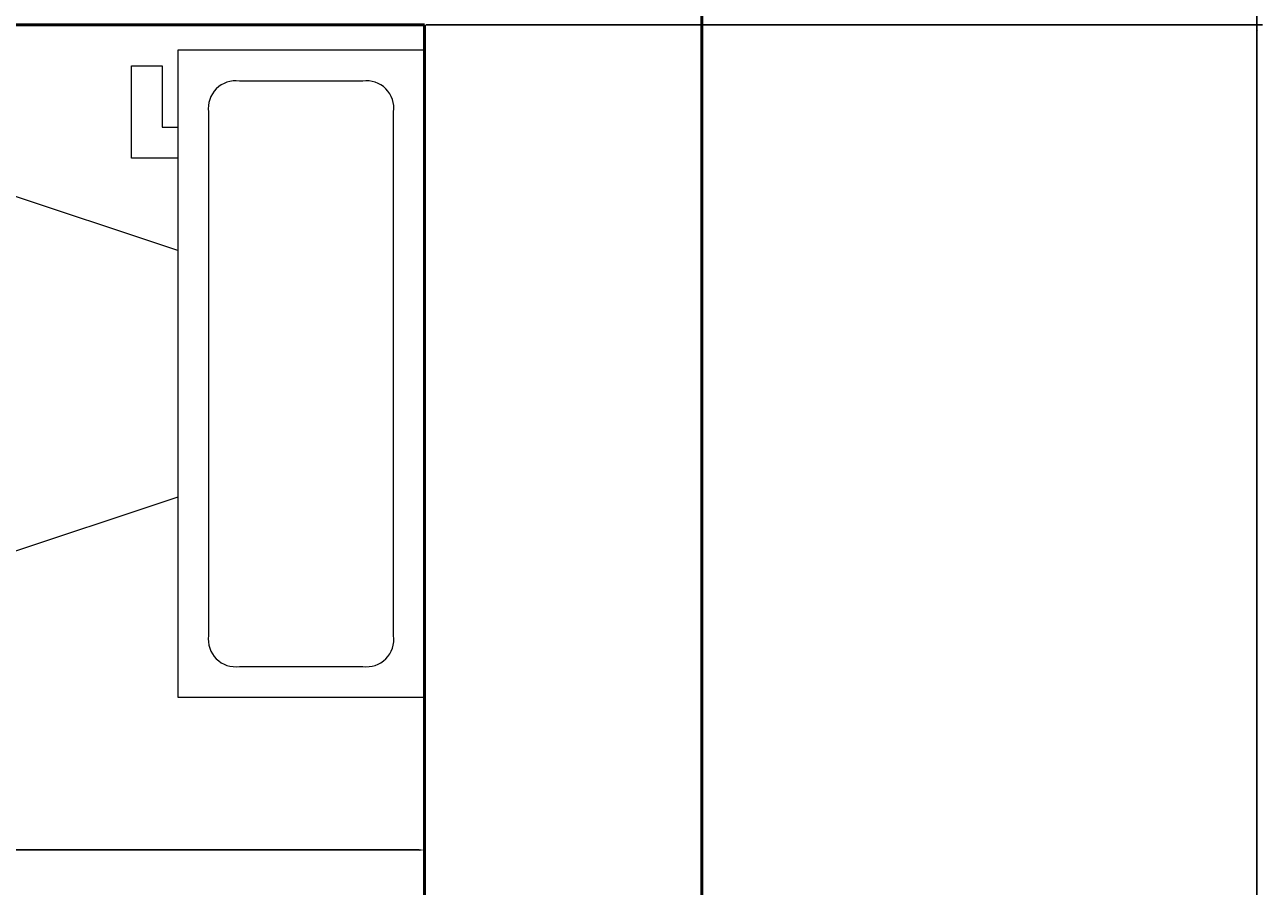
# Model space of a CAD drawing. Units: inches. Extents: x 2621 to 2849, y 2066 to 2463.
# Tile 27 of 28: x 2809 to 2849, y 2407 to 2435. Entities that reach past the tile are written whole.
import ezdxf

# ---------------------------------------------------------------- set-up
doc = ezdxf.new("R2010")
doc.units = ezdxf.units.IN
for name, color, linetype, lineweight in [('A-ANNO-DIMS', 2, 'Continuous', 18), ('A-FLOR-FIXT', 9, 'Continuous', 18), ('A-WALL', 7, 'Continuous', 50)]:
    doc.layers.add(name, color=color, linetype=linetype, lineweight=lineweight)
doc.styles.get("Standard").update_dxf_attribs({"font": 'arial.ttf'})
doc.dimstyles.get("Standard").update_dxf_attribs({"dimtxt": 0.18, "dimasz": 0.18, "dimexe": 0.18, "dimexo": 0.0625, "dimgap": 0.09, "dimtad": 0, "dimtih": 1, "dimtoh": 1, "dimdec": 4, "dimzin": 0, "dimdsep": 46, "dimtxsty": 'Standard', "dimcen": 0.09, "dimadec": 0, "dimazin": 0, "dimtfac": 1, "dimtdec": 4, "dimtofl": 0, "dimtmove": 0, "dimatfit": 3, "dimfxl": 1, "dimtolj": 1, "dimtzin": 0, "dimarcsym": 0})

# ---------------------------------------------------------------- blocks, each defined once
blk = doc.blocks.new('Toilet - top')
for p, q in [((9.5, -6), (9.5, -2)), ((-8, -8.5), (-8, -8)), ((-7, -8), (-7, -9.5)), ((-4, -8), (-6, -14)), ((4, -8), (6, -14)), ((-10, -8.5), (-8, -8.5)), ((-10, -9.5), (-10, -8.5)), ((-7, -9.5), (-10, -9.5)), ((4, -14), (-4, -14))]:
    blk.add_line(p, q)
blk.add_lwpolyline([(10.5, -8), (10.5, 0), (-10.5, 0), (-10.5, -8)], close=True)
for points in [[(8.5, -1), (-8.5, -1)], [(-9.5, -2), (-9.5, -6)], [(-8.5, -7), (8.5, -7)]]:
    blk.add_lwpolyline(points)
for centre, radius, start, end in [((-8.625, -1.875), 0.884, 81.8699, 188.1301), ((8.625, -1.875), 0.884, 351.8699, 98.1301), ((-8.625, -6.125), 0.884, 171.8699, 278.1301), ((8.625, -6.125), 0.884, 261.8699, 8.1301), ((3.52, -21.58), 12.169, 141.4691, 247.9714), ((4.2, -21.817), 11.329, 136.3677, 238.9468), ((-3.519, -21.58), 12.169, 292.0284, 38.5307), ((-4.2, -21.817), 11.329, 301.053, 43.6321), ((0, -27.876), 4, 245.7318, 294.2682), ((0, -29), 4, 254.8605, 285.1395)]:
    blk.add_arc(centre, radius, start, end)
blk = doc.blocks.new('*D27')
at = {"layer": 'A-ANNO-DIMS', "color": 0, "lineweight": -2, "transparency": 16777216}
for p, q in [((2788.824, 2413.484), (2788.824, 2408.409)), ((2821.87, 2413.484), (2821.87, 2408.409)), ((2789.004, 2408.589), (2804.88, 2408.589)), ((2821.69, 2408.589), (2805.814, 2408.589))]:
    blk.add_line(p, q, dxfattribs=at)
at = {"layer": 'A-ANNO-DIMS', "color": 0, "transparency": 16777216}
for points in [[(2789.004, 2408.619), (2789.004, 2408.559), (2788.824, 2408.589)], [(2821.69, 2408.619), (2821.69, 2408.559), (2821.87, 2408.589)]]:
    blk.add_solid(points, dxfattribs=at)
at = {"layer": 'Defpoints', "color": 0, "transparency": 16777216}
for p in [(2788.824, 2413.546), (2821.87, 2413.546), (2821.87, 2408.589)]:
    blk.add_point(p, dxfattribs=at)
at = {"layer": 'A-ANNO-DIMS', "color": 0, "transparency": 16777216, "insert": (2805.347, 2408.589), "char_height": 0.18, "attachment_point": 5}
blk.add_mtext('\\A1;WC 33', dxfattribs=at)
blk = doc.blocks.new('*D36')
at = {"layer": 'A-ANNO-DIMS', "color": 0, "lineweight": -2, "transparency": 16777216}
for p, q in [((2830.933, 2444.375), (2849.054, 2444.375)), ((2848.874, 2444.195), (2848.874, 2264.557)), ((2848.874, 2084.555), (2848.874, 2264.193)), ((2830.933, 2084.375), (2849.054, 2084.375))]:
    blk.add_line(p, q, dxfattribs=at)
at = {"layer": 'A-ANNO-DIMS', "color": 0, "transparency": 16777216}
for points in [[(2848.844, 2444.195), (2848.904, 2444.195), (2848.874, 2444.375)], [(2848.844, 2084.555), (2848.904, 2084.555), (2848.874, 2084.375)]]:
    blk.add_solid(points, dxfattribs=at)
at = {"layer": 'Defpoints', "color": 0, "transparency": 16777216}
for p in [(2830.87, 2444.375), (2848.874, 2444.375), (2830.87, 2084.375)]:
    blk.add_point(p, dxfattribs=at)
at = {"layer": 'A-ANNO-DIMS', "color": 0, "transparency": 16777216, "insert": (2848.874, 2264.375), "char_height": 0.18, "attachment_point": 5}
blk.add_mtext('\\A1;360', dxfattribs=at)
blk = doc.blocks.new('*D48')
at = {"layer": 'A-ANNO-DIMS', "color": 0, "lineweight": -2, "transparency": 16777216}
for p, q in [((2821.933, 2435.375), (2849.054, 2435.375)), ((2848.874, 2435.195), (2848.874, 2405.556)), ((2848.874, 2375.555), (2848.874, 2405.193)), ((2821.933, 2375.375), (2849.054, 2375.375))]:
    blk.add_line(p, q, dxfattribs=at)
at = {"layer": 'A-ANNO-DIMS', "color": 0, "transparency": 16777216}
for points in [[(2848.844, 2435.195), (2848.904, 2435.195), (2848.874, 2435.375)], [(2848.844, 2375.555), (2848.904, 2375.555), (2848.874, 2375.375)]]:
    blk.add_solid(points, dxfattribs=at)
at = {"layer": 'Defpoints', "color": 0, "transparency": 16777216}
for p in [(2821.87, 2435.375), (2848.874, 2435.375), (2821.87, 2375.375)]:
    blk.add_point(p, dxfattribs=at)
at = {"layer": 'A-ANNO-DIMS', "color": 0, "transparency": 16777216, "insert": (2848.874, 2405.375), "char_height": 0.18, "attachment_point": 5}
blk.add_mtext('\\A1;60', dxfattribs=at)

msp = doc.modelspace()

# ---------------------------------------------------------------- linework, layer by layer
at = {"layer": 'A-WALL'}
for p, q in [((2767.8701, 2435.3746), (2821.8701, 2435.3746)), ((2821.8701, 2435.3746), (2821.8701, 2375.3746)), ((2821.8701, 2435.3746), (2821.8701, 2375.3746))]:
    msp.add_line(p, q, dxfattribs=at)
msp.add_lwpolyline([(2761.8701, 2084.3746), (2638.8701, 2084.3746), (2638.8701, 2444.3746), (2830.8701, 2444.3746), (2830.8701, 2084.3746), (2797.8701, 2084.3746)], dxfattribs=at)

# ---------------------------------------------------------------- block references
at = {"layer": 'A-FLOR-FIXT', "rotation": 270}
msp.add_blockref('Toilet - top', (2821.8701, 2424.0461), dxfattribs=at)

# ---------------------------------------------------------------- dimensions: what is measured, and where the dimension line sits
at = {"layer": 'A-ANNO-DIMS'}
for base, p1, p2, picture, middle in [((2848.8736, 2444.3746), (2830.8701, 2084.3746), (2830.8701, 2444.3746), '*D36', (2848.8736, 2264.3746)), ((2848.8736, 2435.3746), (2821.8701, 2375.3746), (2821.8701, 2435.3746), '*D48', (2848.8736, 2405.3746))]:
    dim = msp.add_linear_dim(base=base, p1=p1, p2=p2, angle=90, dimstyle='Standard', override={"dimdec": 0, "dimlfac": 1, "dimrnd": 0, "dimzin": 0, "dimdsep": 46, "dimlunit": 2}, dxfattribs=at)
    dim.commit()
    dim.dimension.update_dxf_attribs({"geometry": picture, "text_midpoint": middle})
dim = msp.add_linear_dim(base=(2821.8701, 2408.5892), p1=(2788.8239, 2413.5461), p2=(2821.8701, 2413.5461), text='WC <>', dimstyle='Standard', override={"dimdec": 0, "dimlfac": 1, "dimrnd": 0, "dimzin": 0, "dimdsep": 46, "dimlunit": 2}, dxfattribs=at)
dim.commit()
dim.dimension.update_dxf_attribs({"geometry": '*D27', "text_midpoint": (2805.347, 2408.5892)})

doc.saveas('drawing.dxf')
